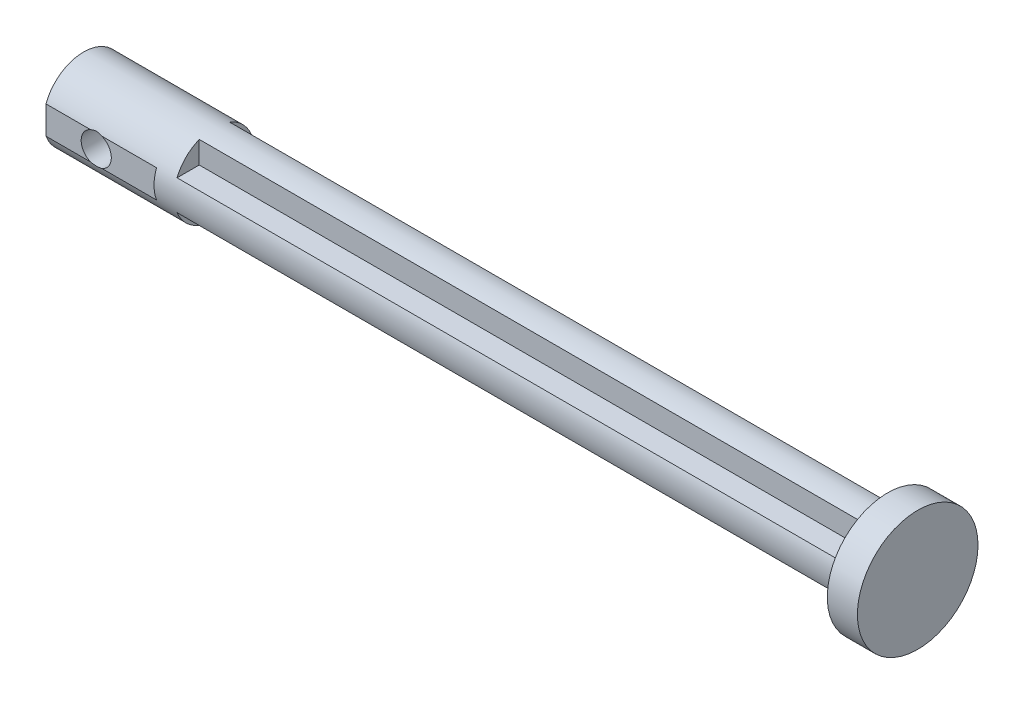
ISO-10303-21;
HEADER;
FILE_DESCRIPTION(('STEP AP214'),'2;1');
FILE_NAME('part.step','',(''),(''),'','','');
FILE_SCHEMA(('AUTOMOTIVE_DESIGN { 1 0 10303 214 1 1 1 1 }'));
ENDSEC;
DATA;
#1=APPLICATION_CONTEXT('core data for automotive mechanical design processes');
#2=APPLICATION_PROTOCOL_DEFINITION('international standard','automotive_design',2000,#1);
#3=PRODUCT_CONTEXT('',#1,'mechanical');
#4=PRODUCT('Part','Part','',(#3));
#5=PRODUCT_RELATED_PRODUCT_CATEGORY('part','',(#4));
#6=PRODUCT_DEFINITION_FORMATION('','',#4);
#7=PRODUCT_DEFINITION_CONTEXT('part definition',#1,'design');
#8=PRODUCT_DEFINITION('design','',#6,#7);
#9=PRODUCT_DEFINITION_SHAPE('','',#8);
#10=(LENGTH_UNIT() NAMED_UNIT(*) SI_UNIT(.MILLI.,.METRE.));
#11=(NAMED_UNIT(*) PLANE_ANGLE_UNIT() SI_UNIT($,.RADIAN.));
#12=(NAMED_UNIT(*) SI_UNIT($,.STERADIAN.) SOLID_ANGLE_UNIT());
#13=UNCERTAINTY_MEASURE_WITH_UNIT(LENGTH_MEASURE(1.E-05),#10,'distance_accuracy_value','');
#14=(GEOMETRIC_REPRESENTATION_CONTEXT(3) GLOBAL_UNCERTAINTY_ASSIGNED_CONTEXT((#13)) GLOBAL_UNIT_ASSIGNED_CONTEXT((#10,
#11,#12)) REPRESENTATION_CONTEXT('',''));
#15=CARTESIAN_POINT('',(0.,0.,0.));
#16=DIRECTION('',(0.,0.,1.));
#17=DIRECTION('',(1.,0.,0.));
#18=AXIS2_PLACEMENT_3D('',#15,#16,#17);
#19=CARTESIAN_POINT('',(80.,0.,0.));
#20=DIRECTION('',(-1.,0.,0.));
#21=DIRECTION('',(0.,0.,1.));
#22=AXIS2_PLACEMENT_3D('',#19,#20,#21);
#23=CYLINDRICAL_SURFACE('',#22,4.);
#24=CARTESIAN_POINT('',(13.,0.,0.));
#25=DIRECTION('',(1.,0.,0.));
#26=DIRECTION('',(0.,0.,-1.));
#27=AXIS2_PLACEMENT_3D('',#24,#25,#26);
#28=CIRCLE('',#27,4.);
#29=CARTESIAN_POINT('',(13.,-1.5,3.70809924354783));
#30=VERTEX_POINT('',#29);
#31=CARTESIAN_POINT('',(13.,-3.70809924354783,1.5));
#32=VERTEX_POINT('',#31);
#33=EDGE_CURVE('E266',#30,#32,#28,.T.);
#34=ORIENTED_EDGE('',*,*,#33,.F.);
#35=DIRECTION('',(1.,0.,0.));
#36=VECTOR('',#35,1.);
#37=CARTESIAN_POINT('',(13.,-1.5,3.70809924354783));
#38=LINE('',#37,#36);
#39=CARTESIAN_POINT('',(80.,-1.5,3.70809924354783));
#40=VERTEX_POINT('',#39);
#41=EDGE_CURVE('E267',#30,#40,#38,.T.);
#42=ORIENTED_EDGE('',*,*,#41,.T.);
#43=CARTESIAN_POINT('',(80.,0.,0.));
#44=DIRECTION('',(1.,0.,0.));
#45=DIRECTION('',(0.,0.,-1.));
#46=AXIS2_PLACEMENT_3D('',#43,#44,#45);
#47=CIRCLE('',#46,4.);
#48=CARTESIAN_POINT('',(80.,1.5,3.70809924354783));
#49=VERTEX_POINT('',#48);
#50=EDGE_CURVE('E302',#49,#40,#47,.T.);
#51=ORIENTED_EDGE('',*,*,#50,.F.);
#52=DIRECTION('',(1.,0.,0.));
#53=VECTOR('',#52,1.);
#54=CARTESIAN_POINT('',(13.,1.5,3.70809924354783));
#55=LINE('',#54,#53);
#56=CARTESIAN_POINT('',(13.,1.5,3.70809924354783));
#57=VERTEX_POINT('',#56);
#58=EDGE_CURVE('E291',#57,#49,#55,.T.);
#59=ORIENTED_EDGE('',*,*,#58,.F.);
#60=CARTESIAN_POINT('',(13.,0.,0.));
#61=DIRECTION('',(1.,0.,0.));
#62=DIRECTION('',(0.,0.,-1.));
#63=AXIS2_PLACEMENT_3D('',#60,#61,#62);
#64=CIRCLE('',#63,4.);
#65=CARTESIAN_POINT('',(13.,3.70809924354783,1.5));
#66=VERTEX_POINT('',#65);
#67=EDGE_CURVE('E283',#66,#57,#64,.T.);
#68=ORIENTED_EDGE('',*,*,#67,.F.);
#69=DIRECTION('',(1.,0.,0.));
#70=VECTOR('',#69,1.);
#71=CARTESIAN_POINT('',(13.,3.70809924354783,1.5));
#72=LINE('',#71,#70);
#73=CARTESIAN_POINT('',(80.,3.70809924354783,1.5));
#74=VERTEX_POINT('',#73);
#75=EDGE_CURVE('E167',#66,#74,#72,.T.);
#76=ORIENTED_EDGE('',*,*,#75,.T.);
#77=CARTESIAN_POINT('',(80.,3.70809924354783,-1.5));
#78=VERTEX_POINT('',#77);
#79=EDGE_CURVE('E174',#78,#74,#47,.T.);
#80=ORIENTED_EDGE('',*,*,#79,.F.);
#81=DIRECTION('',(1.,0.,0.));
#82=VECTOR('',#81,1.);
#83=CARTESIAN_POINT('',(13.,3.70809924354783,-1.5));
#84=LINE('',#83,#82);
#85=CARTESIAN_POINT('',(13.,3.70809924354783,-1.5));
#86=VERTEX_POINT('',#85);
#87=EDGE_CURVE('E312',#86,#78,#84,.T.);
#88=ORIENTED_EDGE('',*,*,#87,.F.);
#89=CARTESIAN_POINT('',(13.,0.,0.));
#90=DIRECTION('',(1.,0.,0.));
#91=DIRECTION('',(0.,0.,-1.));
#92=AXIS2_PLACEMENT_3D('',#89,#90,#91);
#93=CIRCLE('',#92,4.);
#94=CARTESIAN_POINT('',(13.,1.5,-3.70809924354783));
#95=VERTEX_POINT('',#94);
#96=EDGE_CURVE('E319',#95,#86,#93,.T.);
#97=ORIENTED_EDGE('',*,*,#96,.F.);
#98=DIRECTION('',(1.,0.,0.));
#99=VECTOR('',#98,1.);
#100=CARTESIAN_POINT('',(13.,1.5,-3.70809924354783));
#101=LINE('',#100,#99);
#102=CARTESIAN_POINT('',(80.,1.5,-3.70809924354783));
#103=VERTEX_POINT('',#102);
#104=EDGE_CURVE('E341',#95,#103,#101,.T.);
#105=ORIENTED_EDGE('',*,*,#104,.T.);
#106=CARTESIAN_POINT('',(80.,-1.5,-3.70809924354783));
#107=VERTEX_POINT('',#106);
#108=EDGE_CURVE('E169',#107,#103,#47,.T.);
#109=ORIENTED_EDGE('',*,*,#108,.F.);
#110=DIRECTION('',(1.,0.,0.));
#111=VECTOR('',#110,1.);
#112=CARTESIAN_POINT('',(13.,-1.5,-3.70809924354783));
#113=LINE('',#112,#111);
#114=CARTESIAN_POINT('',(13.,-1.5,-3.70809924354783));
#115=VERTEX_POINT('',#114);
#116=EDGE_CURVE('E329',#115,#107,#113,.T.);
#117=ORIENTED_EDGE('',*,*,#116,.F.);
#118=CARTESIAN_POINT('',(13.,0.,0.));
#119=DIRECTION('',(1.,0.,0.));
#120=DIRECTION('',(0.,0.,-1.));
#121=AXIS2_PLACEMENT_3D('',#118,#119,#120);
#122=CIRCLE('',#121,4.);
#123=CARTESIAN_POINT('',(13.,-3.70809924354783,-1.5));
#124=VERTEX_POINT('',#123);
#125=EDGE_CURVE('E342',#124,#115,#122,.T.);
#126=ORIENTED_EDGE('',*,*,#125,.F.);
#127=DIRECTION('',(1.,0.,0.));
#128=VECTOR('',#127,1.);
#129=CARTESIAN_POINT('',(13.,-3.70809924354783,-1.5));
#130=LINE('',#129,#128);
#131=CARTESIAN_POINT('',(80.,-3.70809924354783,-1.5));
#132=VERTEX_POINT('',#131);
#133=EDGE_CURVE('E334',#124,#132,#130,.T.);
#134=ORIENTED_EDGE('',*,*,#133,.T.);
#135=CARTESIAN_POINT('',(80.,-3.70809924354783,1.5));
#136=VERTEX_POINT('',#135);
#137=EDGE_CURVE('E173',#136,#132,#47,.T.);
#138=ORIENTED_EDGE('',*,*,#137,.F.);
#139=DIRECTION('',(1.,0.,0.));
#140=VECTOR('',#139,1.);
#141=CARTESIAN_POINT('',(13.,-3.70809924354783,1.5));
#142=LINE('',#141,#140);
#143=EDGE_CURVE('E272',#32,#136,#142,.T.);
#144=ORIENTED_EDGE('',*,*,#143,.F.);
#145=EDGE_LOOP('',(#34,#42,#51,#59,#68,#76,#80,#88,#97,#105,#109,#117,#126,#134,#138,#144));
#146=FACE_BOUND('',#145,.T.);
#147=DIRECTION('',(-1.,0.,0.));
#148=VECTOR('',#147,1.);
#149=CARTESIAN_POINT('',(80.,1.39194109070751,3.75));
#150=LINE('',#149,#148);
#151=CARTESIAN_POINT('',(11.,1.39194109070751,3.75));
#152=VERTEX_POINT('',#151);
#153=CARTESIAN_POINT('',(5.55901699437495,1.39194109070751,3.75));
#154=VERTEX_POINT('',#153);
#155=EDGE_CURVE('E53',#152,#154,#150,.T.);
#156=ORIENTED_EDGE('',*,*,#155,.F.);
#157=CARTESIAN_POINT('',(11.,0.,0.));
#158=DIRECTION('',(1.,0.,0.));
#159=DIRECTION('',(0.,0.,-1.));
#160=AXIS2_PLACEMENT_3D('',#157,#158,#159);
#161=CIRCLE('',#160,4.);
#162=CARTESIAN_POINT('',(11.,-1.39194109070751,3.75));
#163=VERTEX_POINT('',#162);
#164=EDGE_CURVE('E11',#152,#163,#161,.T.);
#165=ORIENTED_EDGE('',*,*,#164,.T.);
#166=DIRECTION('',(-1.,0.,0.));
#167=VECTOR('',#166,1.);
#168=CARTESIAN_POINT('',(80.,-1.39194109070751,3.75));
#169=LINE('',#168,#167);
#170=CARTESIAN_POINT('',(5.55901699437495,-1.39194109070751,3.75));
#171=VERTEX_POINT('',#170);
#172=EDGE_CURVE('E157',#171,#163,#169,.F.);
#173=ORIENTED_EDGE('',*,*,#172,.F.);
#174=CARTESIAN_POINT('',(6.5,0.,4.));
#175=CARTESIAN_POINT('',(6.50000290230311,-0.0812350589378528,4.00000217456151));
#176=CARTESIAN_POINT('',(6.49338023975162,-0.162450241781792,3.99750379283184));
#177=CARTESIAN_POINT('',(6.46717180473007,-0.322453452352361,3.98778696006928));
#178=CARTESIAN_POINT('',(6.44758789952943,-0.401241827987616,3.98056918893993));
#179=CARTESIAN_POINT('',(6.39624699822824,-0.554060784990878,3.96218832391545));
#180=CARTESIAN_POINT('',(6.36451348317821,-0.628100224162277,3.9510328434944));
#181=CARTESIAN_POINT('',(6.28989358698418,-0.769799310160253,3.92588767765353));
#182=CARTESIAN_POINT('',(6.24700421445584,-0.837457239177879,3.91189723227548));
#183=CARTESIAN_POINT('',(6.14938746892909,-0.967346417045825,3.88186246971217));
#184=CARTESIAN_POINT('',(6.0942697377406,-1.02927073015119,3.86576002583566));
#185=CARTESIAN_POINT('',(5.97458956534116,-1.14324421474363,3.83360220871327));
#186=CARTESIAN_POINT('',(5.91002424391213,-1.19529036359203,3.81754685135033));
#187=CARTESIAN_POINT('',(5.77028253247679,-1.28998202215985,3.78662470617731));
#188=CARTESIAN_POINT('',(5.69479563345418,-1.3321939319576,3.77182648820818));
#189=CARTESIAN_POINT('',(5.53715164583148,-1.40318646334084,3.74599860237433));
#190=CARTESIAN_POINT('',(5.4549972368449,-1.43197244961239,3.73496742975881));
#191=CARTESIAN_POINT('',(5.2898832597418,-1.47408431017549,3.71854412824136));
#192=CARTESIAN_POINT('',(5.20709496156456,-1.48799593218558,3.71293924350838));
#193=CARTESIAN_POINT('',(5.04018384200616,-1.50179556531648,3.70738061461215));
#194=CARTESIAN_POINT('',(4.95606158612553,-1.5016893680263,3.70742453659305));
#195=CARTESIAN_POINT('',(4.79423047478704,-1.48790429610018,3.71297511632055));
#196=CARTESIAN_POINT('',(4.71643909395582,-1.47503808509003,3.71815468871122));
#197=CARTESIAN_POINT('',(4.56421284959468,-1.4374416786833,3.73284938059529));
#198=CARTESIAN_POINT('',(4.48977849338612,-1.41270969663258,3.74236515298863));
#199=CARTESIAN_POINT('',(4.34472293227177,-1.35163748571904,3.76485702190253));
#200=CARTESIAN_POINT('',(4.2742005138787,-1.31508648737101,3.77789517988166));
#201=CARTESIAN_POINT('',(4.14005426240903,-1.23156073762698,3.80594210139319));
#202=CARTESIAN_POINT('',(4.0764328224803,-1.18458238728897,3.82095154457158));
#203=CARTESIAN_POINT('',(3.95339633634912,-1.07781780766549,3.85248038859113));
#204=CARTESIAN_POINT('',(3.89455135925191,-1.01738298716955,3.86903347455671));
#205=CARTESIAN_POINT('',(3.7876620337942,-0.88731259081902,3.90091728164085));
#206=CARTESIAN_POINT('',(3.73961934539433,-0.817675603497363,3.91624781465952));
#207=CARTESIAN_POINT('',(3.65506960293748,-0.669723436992419,3.9442639480908));
#208=CARTESIAN_POINT('',(3.61875241877894,-0.591290713844719,3.95690498259616));
#209=CARTESIAN_POINT('',(3.56001739572996,-0.428836850524583,3.97778718326962));
#210=CARTESIAN_POINT('',(3.53759338343888,-0.344818210845767,3.98603030341493));
#211=CARTESIAN_POINT('',(3.50837721245806,-0.178375243148665,3.99684443228065));
#212=CARTESIAN_POINT('',(3.50081739361749,-0.0961036195622093,3.99969369025686));
#213=CARTESIAN_POINT('',(3.49930893610008,0.0685724752550242,4.00025893700126));
#214=CARTESIAN_POINT('',(3.50535727968322,0.150976912983373,3.99797606386863));
#215=CARTESIAN_POINT('',(3.53031004230867,0.310262048561859,3.98871709772643));
#216=CARTESIAN_POINT('',(3.54871154373709,0.387233328007336,3.98192470962305));
#217=CARTESIAN_POINT('',(3.59718607254732,0.536941754957221,3.96451477091717));
#218=CARTESIAN_POINT('',(3.62726061794804,0.609678350347534,3.9538967228203));
#219=CARTESIAN_POINT('',(3.69918641243948,0.751247765110156,3.92949624407681));
#220=CARTESIAN_POINT('',(3.74135772922339,0.819903083557796,3.91563000209348));
#221=CARTESIAN_POINT('',(3.83591810317156,0.949392711726626,3.88626671564664));
#222=CARTESIAN_POINT('',(3.88831093254515,1.01022412027045,3.87076907009516));
#223=CARTESIAN_POINT('',(4.00540412212428,1.12603079874454,3.8387332949099));
#224=CARTESIAN_POINT('',(4.0706421827727,1.18046154123569,3.82218696503729));
#225=CARTESIAN_POINT('',(4.20965138470766,1.27771050031903,3.79078815746854));
#226=CARTESIAN_POINT('',(4.2834232913885,1.32052767414518,3.77593583194399));
#227=CARTESIAN_POINT('',(4.43801598677231,1.39337773518998,3.74966829822463));
#228=CARTESIAN_POINT('',(4.51886474591044,1.42335685446918,3.73826760328493));
#229=CARTESIAN_POINT('',(4.68500976368782,1.46907883466889,3.72054032891005));
#230=CARTESIAN_POINT('',(4.77030323619812,1.48483050305535,3.71421061057491));
#231=CARTESIAN_POINT('',(4.93701615954111,1.50086347097839,3.70775894792573));
#232=CARTESIAN_POINT('',(5.01833263171689,1.50207331495837,3.70726444523341));
#233=CARTESIAN_POINT('',(5.17994531627616,1.49136715641593,3.71158412745292));
#234=CARTESIAN_POINT('',(5.26024162467158,1.47945239850123,3.71639780898899));
#235=CARTESIAN_POINT('',(5.41504722671655,1.44355815630242,3.73048141585432));
#236=CARTESIAN_POINT('',(5.48965834624534,1.41995798316524,3.73961085376663));
#237=CARTESIAN_POINT('',(5.63390550849442,1.3616969677992,3.76121548297845));
#238=CARTESIAN_POINT('',(5.70354028807014,1.32703332944945,3.77369151995215));
#239=CARTESIAN_POINT('',(5.83982678969763,1.24552075938154,3.80139723903965));
#240=CARTESIAN_POINT('',(5.90613079679991,1.1981283280301,3.81673698440964));
#241=CARTESIAN_POINT('',(6.0301415609712,1.09334485729906,3.84806246757177));
#242=CARTESIAN_POINT('',(6.08784557478675,1.03595064012808,3.86404840943145));
#243=CARTESIAN_POINT('',(6.19620195582184,0.909080396784622,3.89590424609881));
#244=CARTESIAN_POINT('',(6.24630375343467,0.839118644212992,3.91172104900645));
#245=CARTESIAN_POINT('',(6.33402265527656,0.69121322320082,3.94054514457031));
#246=CARTESIAN_POINT('',(6.37163878773637,0.61326893409062,3.95355221851559));
#247=CARTESIAN_POINT('',(6.43437682904833,0.44799908200231,3.9757429260668));
#248=CARTESIAN_POINT('',(6.4588870646019,0.360413422234207,3.98473657158356));
#249=CARTESIAN_POINT('',(6.49169295992068,0.181875733606381,3.99686242179587));
#250=CARTESIAN_POINT('',(6.49999675148732,0.0909254163648584,3.99999756603967));
#251=CARTESIAN_POINT('',(6.5,0.,4.));
#252=B_SPLINE_CURVE_WITH_KNOTS('',3,(#174,#175,#176,#177,#178,#179,#180,#181,#182,#183,#184,
#185,#186,#187,#188,#189,#190,#191,#192,#193,#194,#195,#196,#197,#198,#199,#200,#201,#202,#203,
#204,#205,#206,#207,#208,#209,#210,#211,#212,#213,#214,#215,#216,#217,#218,#219,#220,#221,#222,
#223,#224,#225,#226,#227,#228,#229,#230,#231,#232,#233,#234,#235,#236,#237,#238,#239,#240,#241,
#242,#243,#244,#245,#246,#247,#248,#249,#250,#251),.UNSPECIFIED.,.T.,.F.,(4,2,2,2,2,2,2,2,2,2,2,
2,2,2,2,2,2,2,2,2,2,2,2,2,2,2,2,2,2,2,2,2,2,2,2,2,2,2,4),(0.,0.24336980156056,0.48670454953046,
0.729571369213572,0.972503379609489,1.22473618582715,1.47704604925622,1.73896674501658,
2.00078269352134,2.25185874416901,2.50283106079707,2.73878345119971,2.97477138060589,
3.21522408387018,3.45575990744258,3.71246153335813,3.96920257905066,4.22991375286075,
4.49050899698846,4.73725019635925,4.9839366839052,5.2211443792384,5.45838293254453,
5.702592218596,5.94689180019868,6.20536519455658,6.46386178920141,6.72343066727204,
6.98283874956507,7.22558763480252,7.46831350211259,7.70363142426533,7.93900886656506,
8.18672471884271,8.43451941997062,8.69572329654039,8.95694749805102,9.22948515032042,
9.50188601796127),.UNSPECIFIED.);
#253=CARTESIAN_POINT('',(4.44098300562505,-1.39194109070751,3.75));
#254=VERTEX_POINT('',#253);
#255=EDGE_CURVE('E168',#171,#254,#252,.T.);
#256=ORIENTED_EDGE('',*,*,#255,.T.);
#257=CARTESIAN_POINT('',(0.,-1.39194109070751,3.75));
#258=VERTEX_POINT('',#257);
#259=EDGE_CURVE('E65',#258,#254,#169,.F.);
#260=ORIENTED_EDGE('',*,*,#259,.F.);
#261=CARTESIAN_POINT('',(0.,0.,0.));
#262=DIRECTION('',(1.,0.,0.));
#263=DIRECTION('',(0.,0.,-1.));
#264=AXIS2_PLACEMENT_3D('',#261,#262,#263);
#265=CIRCLE('',#264,4.);
#266=CARTESIAN_POINT('',(0.,1.39194109070751,3.75));
#267=VERTEX_POINT('',#266);
#268=EDGE_CURVE('E161',#258,#267,#265,.T.);
#269=ORIENTED_EDGE('',*,*,#268,.T.);
#270=CARTESIAN_POINT('',(4.44098300562505,1.39194109070751,3.75));
#271=VERTEX_POINT('',#270);
#272=EDGE_CURVE('E152',#271,#267,#150,.T.);
#273=ORIENTED_EDGE('',*,*,#272,.F.);
#274=EDGE_CURVE('E181',#271,#154,#252,.T.);
#275=ORIENTED_EDGE('',*,*,#274,.T.);
#276=EDGE_LOOP('',(#156,#165,#173,#256,#260,#269,#273,#275));
#277=FACE_BOUND('',#276,.T.);
#278=ADVANCED_FACE('F39',(#146,#277),#23,.T.);
#279=CARTESIAN_POINT('',(0.,0.,0.));
#280=DIRECTION('',(1.,0.,0.));
#281=DIRECTION('',(0.,0.,-1.));
#282=AXIS2_PLACEMENT_3D('',#279,#280,#281);
#283=PLANE('',#282);
#284=DIRECTION('',(0.,1.,0.));
#285=VECTOR('',#284,1.);
#286=CARTESIAN_POINT('',(0.,-1.5,3.75));
#287=LINE('',#286,#285);
#288=EDGE_CURVE('E151',#258,#267,#287,.T.);
#289=ORIENTED_EDGE('',*,*,#288,.T.);
#290=ORIENTED_EDGE('',*,*,#268,.F.);
#291=EDGE_LOOP('',(#289,#290));
#292=FACE_BOUND('',#291,.T.);
#293=ADVANCED_FACE('F166',(#292),#283,.F.);
#294=CARTESIAN_POINT('',(5.,0.,0.));
#295=DIRECTION('',(0.,0.,1.));
#296=DIRECTION('',(1.,0.,0.));
#297=AXIS2_PLACEMENT_3D('',#294,#295,#296);
#298=CYLINDRICAL_SURFACE('',#297,1.5);
#299=CARTESIAN_POINT('',(5.,0.,0.));
#300=DIRECTION('',(0.,0.,1.));
#301=DIRECTION('',(1.,0.,0.));
#302=AXIS2_PLACEMENT_3D('',#299,#300,#301);
#303=CIRCLE('',#302,1.5);
#304=CARTESIAN_POINT('',(6.5,0.,0.));
#305=VERTEX_POINT('',#304);
#306=EDGE_CURVE('E376',#305,#305,#303,.T.);
#307=ORIENTED_EDGE('',*,*,#306,.F.);
#308=EDGE_LOOP('',(#307));
#309=FACE_BOUND('',#308,.T.);
#310=CARTESIAN_POINT('',(5.,0.,3.75));
#311=DIRECTION('',(0.,0.,1.));
#312=DIRECTION('',(1.,0.,0.));
#313=AXIS2_PLACEMENT_3D('',#310,#311,#312);
#314=CIRCLE('',#313,1.5);
#315=EDGE_CURVE('E50',#254,#271,#314,.F.);
#316=ORIENTED_EDGE('',*,*,#315,.F.);
#317=ORIENTED_EDGE('',*,*,#255,.F.);
#318=EDGE_CURVE('E190',#154,#171,#314,.F.);
#319=ORIENTED_EDGE('',*,*,#318,.F.);
#320=ORIENTED_EDGE('',*,*,#274,.F.);
#321=EDGE_LOOP('',(#316,#317,#319,#320));
#322=FACE_BOUND('',#321,.T.);
#323=ADVANCED_FACE('F189',(#309,#322),#298,.F.);
#324=CARTESIAN_POINT('',(13.,1.5,1.5));
#325=DIRECTION('',(0.,0.,-1.));
#326=DIRECTION('',(0.,1.,0.));
#327=AXIS2_PLACEMENT_3D('',#324,#325,#326);
#328=PLANE('',#327);
#329=DIRECTION('',(0.,1.,0.));
#330=VECTOR('',#329,1.);
#331=CARTESIAN_POINT('',(80.,1.5,1.5));
#332=LINE('',#331,#330);
#333=CARTESIAN_POINT('',(80.,1.5,1.5));
#334=VERTEX_POINT('',#333);
#335=EDGE_CURVE('E290',#334,#74,#332,.T.);
#336=ORIENTED_EDGE('',*,*,#335,.T.);
#337=ORIENTED_EDGE('',*,*,#75,.F.);
#338=DIRECTION('',(0.,1.,0.));
#339=VECTOR('',#338,1.);
#340=CARTESIAN_POINT('',(13.,1.5,1.5));
#341=LINE('',#340,#339);
#342=CARTESIAN_POINT('',(13.,1.5,1.5));
#343=VERTEX_POINT('',#342);
#344=EDGE_CURVE('E289',#343,#66,#341,.T.);
#345=ORIENTED_EDGE('',*,*,#344,.F.);
#346=DIRECTION('',(1.,0.,0.));
#347=VECTOR('',#346,1.);
#348=CARTESIAN_POINT('',(13.,1.5,1.5));
#349=LINE('',#348,#347);
#350=EDGE_CURVE('E180',#343,#334,#349,.T.);
#351=ORIENTED_EDGE('',*,*,#350,.T.);
#352=EDGE_LOOP('',(#336,#337,#345,#351));
#353=FACE_BOUND('',#352,.T.);
#354=ADVANCED_FACE('F194',(#353),#328,.F.);
#355=CARTESIAN_POINT('',(13.,1.5,3.70809924354783));
#356=DIRECTION('',(0.,-1.,0.));
#357=DIRECTION('',(0.,0.,-1.));
#358=AXIS2_PLACEMENT_3D('',#355,#356,#357);
#359=PLANE('',#358);
#360=DIRECTION('',(0.,0.,-1.));
#361=VECTOR('',#360,1.);
#362=CARTESIAN_POINT('',(80.,1.5,3.70809924354783));
#363=LINE('',#362,#361);
#364=EDGE_CURVE('E295',#49,#334,#363,.T.);
#365=ORIENTED_EDGE('',*,*,#364,.T.);
#366=ORIENTED_EDGE('',*,*,#350,.F.);
#367=DIRECTION('',(0.,0.,-1.));
#368=VECTOR('',#367,1.);
#369=CARTESIAN_POINT('',(13.,1.5,3.70809924354783));
#370=LINE('',#369,#368);
#371=EDGE_CURVE('E286',#57,#343,#370,.T.);
#372=ORIENTED_EDGE('',*,*,#371,.F.);
#373=ORIENTED_EDGE('',*,*,#58,.T.);
#374=EDGE_LOOP('',(#365,#366,#372,#373));
#375=FACE_BOUND('',#374,.T.);
#376=ADVANCED_FACE('F247',(#375),#359,.F.);
#377=CARTESIAN_POINT('',(13.,0.,0.));
#378=DIRECTION('',(1.,0.,0.));
#379=DIRECTION('',(0.,0.,-1.));
#380=AXIS2_PLACEMENT_3D('',#377,#378,#379);
#381=PLANE('',#380);
#382=ORIENTED_EDGE('',*,*,#67,.T.);
#383=ORIENTED_EDGE('',*,*,#371,.T.);
#384=ORIENTED_EDGE('',*,*,#344,.T.);
#385=EDGE_LOOP('',(#382,#383,#384));
#386=FACE_BOUND('',#385,.T.);
#387=ADVANCED_FACE('F218',(#386),#381,.T.);
#388=CARTESIAN_POINT('',(13.,1.5,-1.5));
#389=DIRECTION('',(0.,-1.,0.));
#390=DIRECTION('',(0.,0.,-1.));
#391=AXIS2_PLACEMENT_3D('',#388,#389,#390);
#392=PLANE('',#391);
#393=DIRECTION('',(0.,0.,-1.));
#394=VECTOR('',#393,1.);
#395=CARTESIAN_POINT('',(80.,1.5,-1.5));
#396=LINE('',#395,#394);
#397=CARTESIAN_POINT('',(80.,1.5,-1.5));
#398=VERTEX_POINT('',#397);
#399=EDGE_CURVE('E317',#398,#103,#396,.T.);
#400=ORIENTED_EDGE('',*,*,#399,.T.);
#401=ORIENTED_EDGE('',*,*,#104,.F.);
#402=DIRECTION('',(0.,0.,-1.));
#403=VECTOR('',#402,1.);
#404=CARTESIAN_POINT('',(13.,1.5,-1.5));
#405=LINE('',#404,#403);
#406=CARTESIAN_POINT('',(13.,1.5,-1.5));
#407=VERTEX_POINT('',#406);
#408=EDGE_CURVE('E325',#407,#95,#405,.T.);
#409=ORIENTED_EDGE('',*,*,#408,.F.);
#410=DIRECTION('',(1.,0.,0.));
#411=VECTOR('',#410,1.);
#412=CARTESIAN_POINT('',(13.,1.5,-1.5));
#413=LINE('',#412,#411);
#414=EDGE_CURVE('E367',#407,#398,#413,.T.);
#415=ORIENTED_EDGE('',*,*,#414,.T.);
#416=EDGE_LOOP('',(#400,#401,#409,#415));
#417=FACE_BOUND('',#416,.T.);
#418=ADVANCED_FACE('F211',(#417),#392,.F.);
#419=CARTESIAN_POINT('',(13.,1.5,-1.5));
#420=DIRECTION('',(0.,0.,1.));
#421=DIRECTION('',(0.,-1.,0.));
#422=AXIS2_PLACEMENT_3D('',#419,#420,#421);
#423=PLANE('',#422);
#424=DIRECTION('',(0.,-1.,0.));
#425=VECTOR('',#424,1.);
#426=CARTESIAN_POINT('',(80.,1.5,-1.5));
#427=LINE('',#426,#425);
#428=EDGE_CURVE('E300',#78,#398,#427,.T.);
#429=ORIENTED_EDGE('',*,*,#428,.T.);
#430=ORIENTED_EDGE('',*,*,#414,.F.);
#431=DIRECTION('',(0.,-1.,0.));
#432=VECTOR('',#431,1.);
#433=CARTESIAN_POINT('',(13.,1.5,-1.5));
#434=LINE('',#433,#432);
#435=EDGE_CURVE('E323',#86,#407,#434,.T.);
#436=ORIENTED_EDGE('',*,*,#435,.F.);
#437=ORIENTED_EDGE('',*,*,#87,.T.);
#438=EDGE_LOOP('',(#429,#430,#436,#437));
#439=FACE_BOUND('',#438,.T.);
#440=ADVANCED_FACE('F208',(#439),#423,.F.);
#441=CARTESIAN_POINT('',(13.,0.,0.));
#442=DIRECTION('',(1.,0.,0.));
#443=DIRECTION('',(0.,0.,-1.));
#444=AXIS2_PLACEMENT_3D('',#441,#442,#443);
#445=PLANE('',#444);
#446=ORIENTED_EDGE('',*,*,#96,.T.);
#447=ORIENTED_EDGE('',*,*,#435,.T.);
#448=ORIENTED_EDGE('',*,*,#408,.T.);
#449=EDGE_LOOP('',(#446,#447,#448));
#450=FACE_BOUND('',#449,.T.);
#451=ADVANCED_FACE('F214',(#450),#445,.T.);
#452=CARTESIAN_POINT('',(13.,-3.70809924354783,-1.5));
#453=DIRECTION('',(0.,0.,1.));
#454=DIRECTION('',(0.,-1.,0.));
#455=AXIS2_PLACEMENT_3D('',#452,#453,#454);
#456=PLANE('',#455);
#457=DIRECTION('',(0.,-1.,0.));
#458=VECTOR('',#457,1.);
#459=CARTESIAN_POINT('',(80.,-3.70809924354783,-1.5));
#460=LINE('',#459,#458);
#461=CARTESIAN_POINT('',(80.,-1.5,-1.5));
#462=VERTEX_POINT('',#461);
#463=EDGE_CURVE('E336',#462,#132,#460,.T.);
#464=ORIENTED_EDGE('',*,*,#463,.T.);
#465=ORIENTED_EDGE('',*,*,#133,.F.);
#466=DIRECTION('',(0.,-1.,0.));
#467=VECTOR('',#466,1.);
#468=CARTESIAN_POINT('',(13.,-3.70809924354783,-1.5));
#469=LINE('',#468,#467);
#470=CARTESIAN_POINT('',(13.,-1.5,-1.5));
#471=VERTEX_POINT('',#470);
#472=EDGE_CURVE('E335',#471,#124,#469,.T.);
#473=ORIENTED_EDGE('',*,*,#472,.F.);
#474=DIRECTION('',(1.,0.,0.));
#475=VECTOR('',#474,1.);
#476=CARTESIAN_POINT('',(13.,-1.5,-1.5));
#477=LINE('',#476,#475);
#478=EDGE_CURVE('E332',#471,#462,#477,.T.);
#479=ORIENTED_EDGE('',*,*,#478,.T.);
#480=EDGE_LOOP('',(#464,#465,#473,#479));
#481=FACE_BOUND('',#480,.T.);
#482=ADVANCED_FACE('F225',(#481),#456,.F.);
#483=CARTESIAN_POINT('',(13.,-1.5,-1.5));
#484=DIRECTION('',(0.,1.,0.));
#485=DIRECTION('',(0.,0.,1.));
#486=AXIS2_PLACEMENT_3D('',#483,#484,#485);
#487=PLANE('',#486);
#488=DIRECTION('',(0.,0.,1.));
#489=VECTOR('',#488,1.);
#490=CARTESIAN_POINT('',(80.,-1.5,-1.5));
#491=LINE('',#490,#489);
#492=EDGE_CURVE('E338',#107,#462,#491,.T.);
#493=ORIENTED_EDGE('',*,*,#492,.T.);
#494=ORIENTED_EDGE('',*,*,#478,.F.);
#495=DIRECTION('',(0.,0.,1.));
#496=VECTOR('',#495,1.);
#497=CARTESIAN_POINT('',(13.,-1.5,-1.5));
#498=LINE('',#497,#496);
#499=EDGE_CURVE('E350',#115,#471,#498,.T.);
#500=ORIENTED_EDGE('',*,*,#499,.F.);
#501=ORIENTED_EDGE('',*,*,#116,.T.);
#502=EDGE_LOOP('',(#493,#494,#500,#501));
#503=FACE_BOUND('',#502,.T.);
#504=ADVANCED_FACE('F223',(#503),#487,.F.);
#505=CARTESIAN_POINT('',(13.,0.,0.));
#506=DIRECTION('',(1.,0.,0.));
#507=DIRECTION('',(0.,0.,-1.));
#508=AXIS2_PLACEMENT_3D('',#505,#506,#507);
#509=PLANE('',#508);
#510=ORIENTED_EDGE('',*,*,#125,.T.);
#511=ORIENTED_EDGE('',*,*,#499,.T.);
#512=ORIENTED_EDGE('',*,*,#472,.T.);
#513=EDGE_LOOP('',(#510,#511,#512));
#514=FACE_BOUND('',#513,.T.);
#515=ADVANCED_FACE('F227',(#514),#509,.T.);
#516=CARTESIAN_POINT('',(13.,-1.5,3.70809924354783));
#517=DIRECTION('',(0.,1.,0.));
#518=DIRECTION('',(0.,0.,1.));
#519=AXIS2_PLACEMENT_3D('',#516,#517,#518);
#520=PLANE('',#519);
#521=DIRECTION('',(0.,0.,1.));
#522=VECTOR('',#521,1.);
#523=CARTESIAN_POINT('',(80.,-1.5,3.70809924354783));
#524=LINE('',#523,#522);
#525=CARTESIAN_POINT('',(80.,-1.5,1.5));
#526=VERTEX_POINT('',#525);
#527=EDGE_CURVE('E274',#526,#40,#524,.T.);
#528=ORIENTED_EDGE('',*,*,#527,.T.);
#529=ORIENTED_EDGE('',*,*,#41,.F.);
#530=DIRECTION('',(0.,0.,1.));
#531=VECTOR('',#530,1.);
#532=CARTESIAN_POINT('',(13.,-1.5,3.70809924354783));
#533=LINE('',#532,#531);
#534=CARTESIAN_POINT('',(13.,-1.5,1.5));
#535=VERTEX_POINT('',#534);
#536=EDGE_CURVE('E276',#535,#30,#533,.T.);
#537=ORIENTED_EDGE('',*,*,#536,.F.);
#538=DIRECTION('',(1.,0.,0.));
#539=VECTOR('',#538,1.);
#540=CARTESIAN_POINT('',(13.,-1.5,1.5));
#541=LINE('',#540,#539);
#542=EDGE_CURVE('E352',#535,#526,#541,.T.);
#543=ORIENTED_EDGE('',*,*,#542,.T.);
#544=EDGE_LOOP('',(#528,#529,#537,#543));
#545=FACE_BOUND('',#544,.T.);
#546=ADVANCED_FACE('F234',(#545),#520,.F.);
#547=CARTESIAN_POINT('',(13.,-3.70809924354783,1.5));
#548=DIRECTION('',(0.,0.,-1.));
#549=DIRECTION('',(-1.,0.,0.));
#550=AXIS2_PLACEMENT_3D('',#547,#548,#549);
#551=PLANE('',#550);
#552=DIRECTION('',(0.,1.,0.));
#553=VECTOR('',#552,1.);
#554=CARTESIAN_POINT('',(80.,-3.70809924354783,1.5));
#555=LINE('',#554,#553);
#556=EDGE_CURVE('E280',#136,#526,#555,.T.);
#557=ORIENTED_EDGE('',*,*,#556,.T.);
#558=ORIENTED_EDGE('',*,*,#542,.F.);
#559=DIRECTION('',(0.,1.,0.));
#560=VECTOR('',#559,1.);
#561=CARTESIAN_POINT('',(13.,-3.70809924354783,1.5));
#562=LINE('',#561,#560);
#563=EDGE_CURVE('E273',#32,#535,#562,.T.);
#564=ORIENTED_EDGE('',*,*,#563,.F.);
#565=ORIENTED_EDGE('',*,*,#143,.T.);
#566=EDGE_LOOP('',(#557,#558,#564,#565));
#567=FACE_BOUND('',#566,.T.);
#568=ADVANCED_FACE('F236',(#567),#551,.F.);
#569=CARTESIAN_POINT('',(13.,0.,0.));
#570=DIRECTION('',(1.,0.,0.));
#571=DIRECTION('',(0.,0.,-1.));
#572=AXIS2_PLACEMENT_3D('',#569,#570,#571);
#573=PLANE('',#572);
#574=ORIENTED_EDGE('',*,*,#33,.T.);
#575=ORIENTED_EDGE('',*,*,#563,.T.);
#576=ORIENTED_EDGE('',*,*,#536,.T.);
#577=EDGE_LOOP('',(#574,#575,#576));
#578=FACE_BOUND('',#577,.T.);
#579=ADVANCED_FACE('F204',(#578),#573,.T.);
#580=CARTESIAN_POINT('',(80.,0.,0.));
#581=DIRECTION('',(1.,0.,0.));
#582=DIRECTION('',(0.,0.,-1.));
#583=AXIS2_PLACEMENT_3D('',#580,#581,#582);
#584=PLANE('',#583);
#585=CARTESIAN_POINT('',(80.,0.,0.));
#586=DIRECTION('',(1.,0.,0.));
#587=DIRECTION('',(0.,0.,-1.));
#588=AXIS2_PLACEMENT_3D('',#585,#586,#587);
#589=CIRCLE('',#588,6.);
#590=CARTESIAN_POINT('',(80.,0.,-6.));
#591=VERTEX_POINT('',#590);
#592=EDGE_CURVE('E373',#591,#591,#589,.T.);
#593=ORIENTED_EDGE('',*,*,#592,.F.);
#594=EDGE_LOOP('',(#593));
#595=FACE_BOUND('',#594,.T.);
#596=ORIENTED_EDGE('',*,*,#527,.F.);
#597=ORIENTED_EDGE('',*,*,#556,.F.);
#598=ORIENTED_EDGE('',*,*,#137,.T.);
#599=ORIENTED_EDGE('',*,*,#463,.F.);
#600=ORIENTED_EDGE('',*,*,#492,.F.);
#601=ORIENTED_EDGE('',*,*,#108,.T.);
#602=ORIENTED_EDGE('',*,*,#399,.F.);
#603=ORIENTED_EDGE('',*,*,#428,.F.);
#604=ORIENTED_EDGE('',*,*,#79,.T.);
#605=ORIENTED_EDGE('',*,*,#335,.F.);
#606=ORIENTED_EDGE('',*,*,#364,.F.);
#607=ORIENTED_EDGE('',*,*,#50,.T.);
#608=EDGE_LOOP('',(#596,#597,#598,#599,#600,#601,#602,#603,#604,#605,#606,#607));
#609=FACE_BOUND('',#608,.T.);
#610=ADVANCED_FACE('F205',(#595,#609),#584,.F.);
#611=CARTESIAN_POINT('',(83.,0.,0.));
#612=DIRECTION('',(-1.,0.,0.));
#613=DIRECTION('',(0.,0.,1.));
#614=AXIS2_PLACEMENT_3D('',#611,#612,#613);
#615=CYLINDRICAL_SURFACE('',#614,6.);
#616=CARTESIAN_POINT('',(83.,0.,0.));
#617=DIRECTION('',(1.,0.,0.));
#618=DIRECTION('',(0.,0.,-1.));
#619=AXIS2_PLACEMENT_3D('',#616,#617,#618);
#620=CIRCLE('',#619,6.);
#621=CARTESIAN_POINT('',(83.,0.,-6.));
#622=VERTEX_POINT('',#621);
#623=EDGE_CURVE('E354',#622,#622,#620,.T.);
#624=ORIENTED_EDGE('',*,*,#623,.F.);
#625=EDGE_LOOP('',(#624));
#626=FACE_BOUND('',#625,.T.);
#627=ORIENTED_EDGE('',*,*,#592,.T.);
#628=EDGE_LOOP('',(#627));
#629=FACE_BOUND('',#628,.T.);
#630=ADVANCED_FACE('F199',(#626,#629),#615,.T.);
#631=CARTESIAN_POINT('',(83.,0.,0.));
#632=DIRECTION('',(1.,0.,0.));
#633=DIRECTION('',(0.,0.,-1.));
#634=AXIS2_PLACEMENT_3D('',#631,#632,#633);
#635=PLANE('',#634);
#636=ORIENTED_EDGE('',*,*,#623,.T.);
#637=EDGE_LOOP('',(#636));
#638=FACE_BOUND('',#637,.T.);
#639=ADVANCED_FACE('F200',(#638),#635,.T.);
#640=CARTESIAN_POINT('',(5.,0.,0.));
#641=DIRECTION('',(0.,0.,1.));
#642=DIRECTION('',(1.,0.,0.));
#643=AXIS2_PLACEMENT_3D('',#640,#641,#642);
#644=PLANE('',#643);
#645=ORIENTED_EDGE('',*,*,#306,.T.);
#646=EDGE_LOOP('',(#645));
#647=FACE_BOUND('',#646,.T.);
#648=ADVANCED_FACE('F193',(#647),#644,.T.);
#649=CARTESIAN_POINT('',(0.,0.,3.75));
#650=DIRECTION('',(0.,0.,1.));
#651=DIRECTION('',(1.,0.,0.));
#652=AXIS2_PLACEMENT_3D('',#649,#650,#651);
#653=PLANE('',#652);
#654=ORIENTED_EDGE('',*,*,#155,.T.);
#655=ORIENTED_EDGE('',*,*,#318,.T.);
#656=ORIENTED_EDGE('',*,*,#172,.T.);
#657=DIRECTION('',(0.,1.,0.));
#658=VECTOR('',#657,1.);
#659=CARTESIAN_POINT('',(11.,-1.5,3.75));
#660=LINE('',#659,#658);
#661=EDGE_CURVE('E158',#163,#152,#660,.T.);
#662=ORIENTED_EDGE('',*,*,#661,.T.);
#663=EDGE_LOOP('',(#654,#655,#656,#662));
#664=FACE_BOUND('',#663,.T.);
#665=ADVANCED_FACE('F384',(#664),#653,.T.);
#666=CARTESIAN_POINT('',(11.,-1.5,3.75));
#667=DIRECTION('',(1.,0.,0.));
#668=DIRECTION('',(0.,0.,-1.));
#669=AXIS2_PLACEMENT_3D('',#666,#667,#668);
#670=PLANE('',#669);
#671=ORIENTED_EDGE('',*,*,#661,.F.);
#672=ORIENTED_EDGE('',*,*,#164,.F.);
#673=EDGE_LOOP('',(#671,#672));
#674=FACE_BOUND('',#673,.T.);
#675=ADVANCED_FACE('F390',(#674),#670,.F.);
#676=ORIENTED_EDGE('',*,*,#272,.T.);
#677=ORIENTED_EDGE('',*,*,#288,.F.);
#678=ORIENTED_EDGE('',*,*,#259,.T.);
#679=ORIENTED_EDGE('',*,*,#315,.T.);
#680=EDGE_LOOP('',(#676,#677,#678,#679));
#681=FACE_BOUND('',#680,.T.);
#682=ADVANCED_FACE('F155',(#681),#653,.T.);
#683=CLOSED_SHELL('',(#278,#293,#323,#354,#376,#387,#418,#440,#451,#482,#504,#515,#546,#568,
#579,#610,#630,#639,#648,#665,#675,#682));
#684=MANIFOLD_SOLID_BREP('B2',#683);
#685=ADVANCED_BREP_SHAPE_REPRESENTATION('',(#18,#684),#14);
#686=SHAPE_DEFINITION_REPRESENTATION(#9,#685);
ENDSEC;
END-ISO-10303-21;
